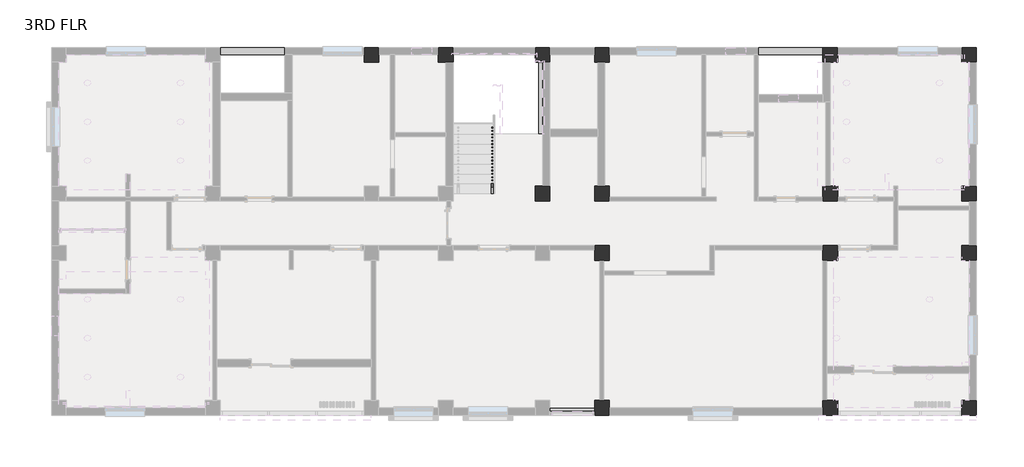
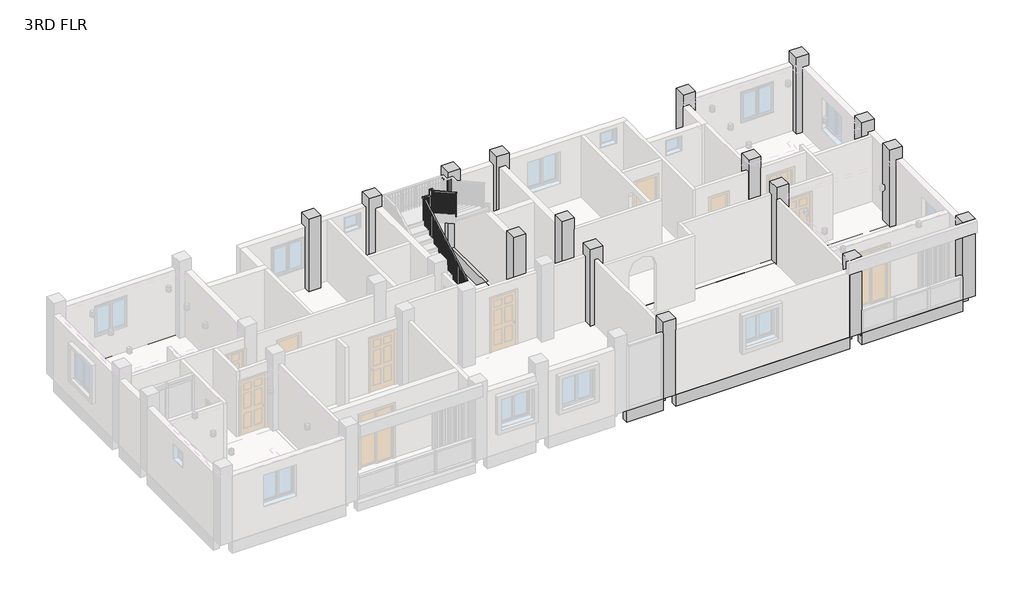
# One storey, part 4 of 5: 29 beams, 16 columns, 1 railing.
"""IFC4 building model written with IfcOpenShell, lengths in millimetres."""

from ifc_helpers import new_model, si_unit, frame, origin, place, context, project, spatial, polyline, outline, extrude, faceted_brep, element, save

model = new_model("IFC4")

# Units and contexts
model_context = context("Model", 3, world=origin())
ifc_project = project(units=[si_unit("LENGTHUNIT", "METRE", prefix="MILLI")], contexts=[model_context])

# Site, building, storey
site = spatial("IfcSite", under=ifc_project)
building = spatial("IfcBuilding", under=site)
storey = spatial("IfcBuildingStorey", under=building, Name="3RD FLR", Elevation=9448.8)

# Beams
placement = place(None, origin())
element("IfcBeam", 1, ObjectType="Concrete-Rectangular Beam : 9\" X 18\" BEAM", at=placement, inside=storey, context=model_context, shape_type="SweptSolid", body=[
    extrude(outline(polyline([(1310.3916602, -10887.8679047), (1310.3916602, -11116.4679047), (-61.2083398, -11116.4679047), (-61.2083398, -10887.8679047), (1310.3916602, -10887.8679047)])), frame((0.0, 0.0, 8991.6), z_axis=(0.0, 0.0, 1.0), x_axis=(1.0, 0.0, 0.0)), (0.0, 0.0, 1.0), 457.2),
])
element("IfcBeam", 2, ObjectType="Concrete-Rectangular Beam : 9\" X 18\" BEAM", at=placement, inside=storey, context=model_context, shape_type="SweptSolid", body=[
    extrude(outline(polyline([(1424.6916602, -6358.3794704), (1653.2916602, -6358.3794704), (1653.2916602, -10659.2679047), (1424.6916602, -10659.2679047), (1424.6916602, -6358.3794704)])), frame((0.0, 0.0, 8991.6), z_axis=(0.0, 0.0, 1.0), x_axis=(1.0, 0.0, 0.0)), (0.0, 0.0, 1.0), 457.2),
])
element("IfcBeam", 3, ObjectType="Concrete-Rectangular Beam : 9\" X 18\" BEAM", at=placement, inside=storey, context=model_context, shape_type="SweptSolid", body=[
    extrude(outline(polyline([(1424.6916602, -4529.5794704), (1653.2916602, -4529.5794704), (1653.2916602, -5901.1794704), (1424.6916602, -5901.1794704), (1424.6916602, -4529.5794704)])), frame((0.0, 0.0, 8991.6), z_axis=(0.0, 0.0, 1.0), x_axis=(1.0, 0.0, 0.0)), (0.0, 0.0, 1.0), 457.2),
])
element("IfcBeam", 4, ObjectType="Concrete-Rectangular Beam : 9\" X 18\" BEAM", at=placement, inside=storey, context=model_context, shape_type="SweptSolid", body=[
    extrude(outline(polyline([(8317.2128058, -10887.8679047), (8317.2128058, -11116.4679047), (1767.5916602, -11116.4679047), (1767.5916602, -10887.8679047), (8317.2128058, -10887.8679047)])), frame((0.0, 0.0, 8991.6), z_axis=(0.0, 0.0, 1.0), x_axis=(1.0, 0.0, 0.0)), (0.0, 0.0, 1.0), 457.2),
])
element("IfcBeam", 5, ObjectType="Concrete-Rectangular Beam : 9\" X 18\" BEAM", at=placement, inside=storey, context=model_context, shape_type="SweptSolid", body=[
    extrude(outline(polyline([(12584.4128058, -10887.8679047), (12584.4128058, -11116.4679047), (8774.4128058, -11116.4679047), (8774.4128058, -10887.8679047), (12584.4128058, -10887.8679047)])), frame((0.0, 0.0, 8991.6), z_axis=(0.0, 0.0, 1.0), x_axis=(1.0, 0.0, 0.0)), (0.0, 0.0, 1.0), 457.2),
])
element("IfcBeam", 6, ObjectType="Concrete-Rectangular Beam : 9\" X 18\" BEAM", at=placement, inside=storey, context=model_context, shape_type="SweptSolid", body=[
    extrude(outline(polyline([(12813.0128058, -6358.3794704), (13041.6128058, -6358.3794704), (13041.6128058, -10659.2679047), (12813.0128058, -10659.2679047), (12813.0128058, -6358.3794704)])), frame((0.0, 0.0, 8991.6), z_axis=(0.0, 0.0, 1.0), x_axis=(1.0, 0.0, 0.0)), (0.0, 0.0, 1.0), 457.2),
])
element("IfcBeam", 7, ObjectType="Concrete-Rectangular Beam : 9\" X 18\" BEAM", at=placement, inside=storey, context=model_context, shape_type="SweptSolid", body=[
    extrude(outline(polyline([(12813.0128058, -4529.5794704), (13041.6128058, -4529.5794704), (13041.6128058, -5901.1794704), (12813.0128058, -5901.1794704), (12813.0128058, -4529.5794704)])), frame((0.0, 0.0, 8991.6), z_axis=(0.0, 0.0, 1.0), x_axis=(1.0, 0.0, 0.0)), (0.0, 0.0, 1.0), 457.2),
])
element("IfcBeam", 8, ObjectType="Concrete-Rectangular Beam : 9\" X 18\" BEAM", at=placement, inside=storey, context=model_context, shape_type="SweptSolid", body=[
    extrude(outline(polyline([(12813.0128058, -262.3794704), (13041.6128058, -262.3794704), (13041.6128058, -4072.3794704), (12813.0128058, -4072.3794704), (12813.0128058, -262.3794704)])), frame((0.0, 0.0, 8991.6), z_axis=(0.0, 0.0, 1.0), x_axis=(1.0, 0.0, 0.0)), (0.0, 0.0, 1.0), 457.2),
])
element("IfcBeam", 9, ObjectType="Concrete-Rectangular Beam : 9\" X 18\" BEAM", at=placement, inside=storey, context=model_context, shape_type="SweptSolid", body=[
    extrude(outline(polyline([(8774.4128058, -33.7794704), (8774.4128058, 194.8205296), (12584.4128058, 194.8205296), (12584.4128058, -33.7794704), (8774.4128058, -33.7794704)])), frame((0.0, 0.0, 8991.6), z_axis=(0.0, 0.0, 1.0), x_axis=(1.0, 0.0, 0.0)), (0.0, 0.0, 1.0), 457.2),
])
element("IfcBeam", 10, ObjectType="Concrete-Rectangular Beam : 9\" X 18\" BEAM", at=placement, inside=storey, context=model_context, shape_type="SweptSolid", body=[
    extrude(outline(polyline([(1767.5916602, -33.7794704), (1767.5916602, 194.8205296), (8317.2128058, 194.8205296), (8317.2128058, -33.7794704), (1767.5916602, -33.7794704)])), frame((0.0, 0.0, 8991.6), z_axis=(0.0, 0.0, 1.0), x_axis=(1.0, 0.0, 0.0)), (0.0, 0.0, 1.0), 457.2),
])
element("IfcBeam", 11, ObjectType="Concrete-Rectangular Beam : 9\" X 18\" BEAM", at=placement, inside=storey, context=model_context, shape_type="SweptSolid", body=[
    extrude(outline(polyline([(-61.2083398, -33.7794704), (-61.2083398, 194.8205296), (1310.3916602, 194.8205296), (1310.3916602, -33.7794704), (-61.2083398, -33.7794704)])), frame((0.0, 0.0, 8991.6), z_axis=(0.0, 0.0, 1.0), x_axis=(1.0, 0.0, 0.0)), (0.0, 0.0, 1.0), 457.2),
])
element("IfcBeam", 12, ObjectType="Concrete-Rectangular Beam : 9\" X 18\" BEAM", at=placement, inside=storey, context=model_context, shape_type="SweptSolid", body=[
    extrude(outline(polyline([(-3029.5456086, -33.7794704), (-3029.5456086, 194.8205296), (-518.4083398, 194.8205296), (-518.4083398, -33.7794704), (-3029.5456086, -33.7794704)])), frame((0.0, 0.0, 8991.6), z_axis=(0.0, 0.0, 1.0), x_axis=(1.0, 0.0, 0.0)), (0.0, 0.0, 1.0), 457.2),
])
element("IfcBeam", 13, ObjectType="Concrete-Rectangular Beam : 9\" X 18\" BEAM", at=placement, inside=storey, context=model_context, shape_type="SweptSolid", body=[
    extrude(outline(polyline([(-5315.5456086, -33.7794704), (-5315.5456086, 194.8205296), (-3486.7456086, 194.8205296), (-3486.7456086, -33.7794704), (-5315.5456086, -33.7794704)])), frame((0.0, 0.0, 8991.6), z_axis=(0.0, 0.0, 1.0), x_axis=(1.0, 0.0, 0.0)), (0.0, 0.0, 1.0), 457.2),
])
element("IfcBeam", 14, ObjectType="Concrete-Rectangular Beam : 9\" X 18\" BEAM", at=placement, inside=storey, context=model_context, shape_type="SweptSolid", body=[
    extrude(outline(polyline([(-10192.3456086, -33.7794704), (-10192.3456086, 194.8205296), (-5772.7456086, 194.8205296), (-5772.7456086, -33.7794704), (-10192.3456086, -33.7794704)])), frame((0.0, 0.0, 8991.6), z_axis=(0.0, 0.0, 1.0), x_axis=(1.0, 0.0, 0.0)), (0.0, 0.0, 1.0), 457.2),
])
element("IfcBeam", 15, ObjectType="Concrete-Rectangular Beam : 9\" X 18\" BEAM", at=placement, inside=storey, context=model_context, shape_type="SweptSolid", body=[
    extrude(outline(polyline([(-14916.7456086, -33.7794704), (-14916.7456086, 194.8205296), (-10649.5456086, 194.8205296), (-10649.5456086, -33.7794704), (-14916.7456086, -33.7794704)])), frame((0.0, 0.0, 8991.6), z_axis=(0.0, 0.0, 1.0), x_axis=(1.0, 0.0, 0.0)), (0.0, 0.0, 1.0), 457.2),
])
element("IfcBeam", 16, ObjectType="Concrete-Rectangular Beam : 9\" X 18\" BEAM", at=placement, inside=storey, context=model_context, shape_type="SweptSolid", body=[
    extrude(outline(polyline([(-518.4083398, -4186.6794704), (-518.4083398, -4415.2794704), (-3029.5456086, -4415.2794704), (-3029.5456086, -4186.6794704), (-518.4083398, -4186.6794704)])), frame((0.0, 0.0, 8991.6), z_axis=(0.0, 0.0, 1.0), x_axis=(1.0, 0.0, 0.0)), (0.0, 0.0, 1.0), 457.2),
])
element("IfcBeam", 17, ObjectType="Concrete-Rectangular Beam : 9\" X 18\" BEAM", at=placement, inside=storey, context=model_context, shape_type="SweptSolid", body=[
    extrude(outline(polyline([(1310.3916602, -4186.6794704), (1310.3916602, -4415.2794704), (-61.2083398, -4415.2794704), (-61.2083398, -4186.6794704), (1310.3916602, -4186.6794704)])), frame((0.0, 0.0, 8991.6), z_axis=(0.0, 0.0, 1.0), x_axis=(1.0, 0.0, 0.0)), (0.0, 0.0, 1.0), 457.2),
])
element("IfcBeam", 18, ObjectType="Concrete-Rectangular Beam : 9\" X 18\" BEAM", at=placement, inside=storey, context=model_context, shape_type="SweptSolid", body=[
    extrude(outline(polyline([(1424.6916602, -262.3794704), (1653.2916602, -262.3794704), (1653.2916602, -4072.3794704), (1424.6916602, -4072.3794704), (1424.6916602, -262.3794704)])), frame((0.0, 0.0, 8991.6), z_axis=(0.0, 0.0, 1.0), x_axis=(1.0, 0.0, 0.0)), (0.0, 0.0, 1.0), 457.2),
])
element("IfcBeam", 19, ObjectType="Concrete-Rectangular Beam : 9\" X 18\" BEAM", at=placement, inside=storey, context=model_context, shape_type="SweptSolid", body=[
    extrude(outline(polyline([(-175.5083398, -4072.3794704), (-404.1083398, -4072.3794704), (-404.1083398, -262.3794704), (-175.5083398, -262.3794704), (-175.5083398, -4072.3794704)])), frame((0.0, 0.0, 8991.6), z_axis=(0.0, 0.0, 1.0), x_axis=(1.0, 0.0, 0.0)), (0.0, 0.0, 1.0), 457.2),
])
element("IfcBeam", 20, ObjectType="Concrete-Rectangular Beam : 9\" X 18\" BEAM", at=placement, inside=storey, context=model_context, shape_type="SweptSolid", body=[
    extrude(outline(polyline([(-3143.8456086, -4072.3794704), (-3372.4456086, -4072.3794704), (-3372.4456086, -262.3794704), (-3143.8456086, -262.3794704), (-3143.8456086, -4072.3794704)])), frame((0.0, 0.0, 8991.6), z_axis=(0.0, 0.0, 1.0), x_axis=(1.0, 0.0, 0.0)), (0.0, 0.0, 1.0), 457.2),
])
element("IfcBeam", 21, ObjectType="Concrete-Rectangular Beam : 9\" X 18\" BEAM", at=placement, inside=storey, context=model_context, shape_type="SweptSolid", body=[
    extrude(outline(polyline([(-5429.8456086, -4072.3794704), (-5658.4456086, -4072.3794704), (-5658.4456086, -262.3794704), (-5429.8456086, -262.3794704), (-5429.8456086, -4072.3794704)])), frame((0.0, 0.0, 8991.6), z_axis=(0.0, 0.0, 1.0), x_axis=(1.0, 0.0, 0.0)), (0.0, 0.0, 1.0), 457.2),
])
element("IfcBeam", 22, ObjectType="Concrete-Rectangular Beam : 9\" X 18\" BEAM", at=placement, inside=storey, context=model_context, shape_type="SweptSolid", body=[
    extrude(outline(polyline([(1310.3916602, -6015.4794704), (1310.3916602, -6244.0794704), (-61.2083398, -6244.0794704), (-61.2083398, -6015.4794704), (1310.3916602, -6015.4794704)])), frame((0.0, 0.0, 8991.6), z_axis=(0.0, 0.0, 1.0), x_axis=(1.0, 0.0, 0.0)), (0.0, 0.0, 1.0), 457.2),
])
element("IfcBeam", 23, ObjectType="Concrete-Rectangular Beam : 9\" X 18\" BEAM", at=placement, inside=storey, context=model_context, shape_type="SweptSolid", body=[
    extrude(outline(polyline([(8317.2128058, -4186.6794704), (8317.2128058, -4415.2794704), (1767.5916602, -4415.2794704), (1767.5916602, -4186.6794704), (8317.2128058, -4186.6794704)])), frame((0.0, 0.0, 8991.6), z_axis=(0.0, 0.0, 1.0), x_axis=(1.0, 0.0, 0.0)), (0.0, 0.0, 1.0), 457.2),
])
element("IfcBeam", 24, ObjectType="Concrete-Rectangular Beam : 9\" X 18\" BEAM", at=placement, inside=storey, context=model_context, shape_type="SweptSolid", body=[
    extrude(outline(polyline([(12584.4128058, -4186.6794704), (12584.4128058, -4415.2794704), (8774.4128058, -4415.2794704), (8774.4128058, -4186.6794704), (12584.4128058, -4186.6794704)])), frame((0.0, 0.0, 8991.6), z_axis=(0.0, 0.0, 1.0), x_axis=(1.0, 0.0, 0.0)), (0.0, 0.0, 1.0), 457.2),
])
element("IfcBeam", 25, ObjectType="Concrete-Rectangular Beam : 9\" X 18\" BEAM", at=placement, inside=storey, context=model_context, shape_type="SweptSolid", body=[
    extrude(outline(polyline([(8774.4128058, -6244.0794704), (8774.4128058, -6015.4794704), (12584.4128058, -6015.4794704), (12584.4128058, -6244.0794704), (8774.4128058, -6244.0794704)])), frame((0.0, 0.0, 8991.6), z_axis=(0.0, 0.0, 1.0), x_axis=(1.0, 0.0, 0.0)), (0.0, 0.0, 1.0), 457.2),
])
element("IfcBeam", 26, ObjectType="Concrete-Rectangular Beam : 9\" X 18\" BEAM", at=placement, inside=storey, context=model_context, shape_type="SweptSolid", body=[
    extrude(outline(polyline([(1767.5916602, -6244.0794704), (1767.5916602, -6015.4794704), (8317.2128058, -6015.4794704), (8317.2128058, -6244.0794704), (1767.5916602, -6244.0794704)])), frame((0.0, 0.0, 8991.6), z_axis=(0.0, 0.0, 1.0), x_axis=(1.0, 0.0, 0.0)), (0.0, 0.0, 1.0), 457.2),
])
element("IfcBeam", 27, ObjectType="Concrete-Rectangular Beam : 9\" X 18\" BEAM", at=placement, inside=storey, context=model_context, shape_type="SweptSolid", body=[
    extrude(outline(polyline([(8431.5128058, -6358.3794704), (8660.1128058, -6358.3794704), (8660.1128058, -10659.2679047), (8431.5128058, -10659.2679047), (8431.5128058, -6358.3794704)])), frame((0.0, 0.0, 8991.6), z_axis=(0.0, 0.0, 1.0), x_axis=(1.0, 0.0, 0.0)), (0.0, 0.0, 1.0), 457.2),
])
element("IfcBeam", 28, ObjectType="Concrete-Rectangular Beam : 9\" X 18\" BEAM", at=placement, inside=storey, context=model_context, shape_type="SweptSolid", body=[
    extrude(outline(polyline([(8431.5128058, -4529.5794704), (8660.1128058, -4529.5794704), (8660.1128058, -5901.1794704), (8431.5128058, -5901.1794704), (8431.5128058, -4529.5794704)])), frame((0.0, 0.0, 8991.6), z_axis=(0.0, 0.0, 1.0), x_axis=(1.0, 0.0, 0.0)), (0.0, 0.0, 1.0), 457.2),
])
element("IfcBeam", 29, ObjectType="Concrete-Rectangular Beam : 9\" X 18\" BEAM", at=placement, inside=storey, context=model_context, shape_type="SweptSolid", body=[
    extrude(outline(polyline([(8431.5128058, -262.3794704), (8660.1128058, -262.3794704), (8660.1128058, -4072.3794704), (8431.5128058, -4072.3794704), (8431.5128058, -262.3794704)])), frame((0.0, 0.0, 8991.6), z_axis=(0.0, 0.0, 1.0), x_axis=(1.0, 0.0, 0.0)), (0.0, 0.0, 1.0), 457.2),
])

# Columns
element("IfcColumn", 30, ObjectType="Concrete-Rectangular-Column : COLUMN 18\" X 18\"", at=placement, inside=storey, context=model_context, shape_type="SweptSolid", body=[
    extrude(outline(polyline([(-5315.5456086, 194.8205296), (-5315.5456086, -262.3794704), (-5772.7456086, -262.3794704), (-5772.7456086, 194.8205296), (-5315.5456086, 194.8205296)])), frame((0.0, 0.0, 9448.8), z_axis=(0.0, 0.0, 1.0), x_axis=(1.0, 0.0, 0.0)), (0.0, 0.0, 1.0), 3048.0),
])
element("IfcColumn", 31, ObjectType="Concrete-Rectangular-Column : COLUMN 18\" X 18\"", at=placement, inside=storey, context=model_context, shape_type="SweptSolid", body=[
    extrude(outline(polyline([(-3029.5456086, 194.8205296), (-3029.5456086, -262.3794704), (-3486.7456086, -262.3794704), (-3486.7456086, 194.8205296), (-3029.5456086, 194.8205296)])), frame((0.0, 0.0, 9448.8), z_axis=(0.0, 0.0, 1.0), x_axis=(1.0, 0.0, 0.0)), (0.0, 0.0, 1.0), 3048.0),
])
element("IfcColumn", 32, ObjectType="Concrete-Rectangular-Column : COLUMN 18\" X 18\"", at=placement, inside=storey, context=model_context, shape_type="SweptSolid", body=[
    extrude(outline(polyline([(-61.2083398, 194.8205296), (-61.2083398, -262.3794704), (-518.4083398, -262.3794704), (-518.4083398, 194.8205296), (-61.2083398, 194.8205296)])), frame((0.0, 0.0, 9448.8), z_axis=(0.0, 0.0, 1.0), x_axis=(1.0, 0.0, 0.0)), (0.0, 0.0, 1.0), 3048.0),
])
element("IfcColumn", 33, ObjectType="Concrete-Rectangular-Column : COLUMN 18\" X 18\"", at=placement, inside=storey, context=model_context, shape_type="SweptSolid", body=[
    extrude(outline(polyline([(1767.5916602, 194.8205296), (1767.5916602, -262.3794704), (1310.3916602, -262.3794704), (1310.3916602, 194.8205296), (1767.5916602, 194.8205296)])), frame((0.0, 0.0, 9448.8), z_axis=(0.0, 0.0, 1.0), x_axis=(1.0, 0.0, 0.0)), (0.0, 0.0, 1.0), 3048.0),
])
element("IfcColumn", 34, ObjectType="Concrete-Rectangular-Column : COLUMN 18\" X 18\"", at=placement, inside=storey, context=model_context, shape_type="SweptSolid", body=[
    extrude(outline(polyline([(8774.4128058, 194.8205296), (8774.4128058, -262.3794704), (8317.2128058, -262.3794704), (8317.2128058, 194.8205296), (8774.4128058, 194.8205296)])), frame((0.0, 0.0, 9448.8), z_axis=(0.0, 0.0, 1.0), x_axis=(1.0, 0.0, 0.0)), (0.0, 0.0, 1.0), 3048.0),
])
element("IfcColumn", 35, ObjectType="Concrete-Rectangular-Column : COLUMN 18\" X 18\"", at=placement, inside=storey, context=model_context, shape_type="SweptSolid", body=[
    extrude(outline(polyline([(13041.6128058, 194.8205296), (13041.6128058, -262.3794704), (12584.4128058, -262.3794704), (12584.4128058, 194.8205296), (13041.6128058, 194.8205296)])), frame((0.0, 0.0, 9448.8), z_axis=(0.0, 0.0, 1.0), x_axis=(1.0, 0.0, 0.0)), (0.0, 0.0, 1.0), 3048.0),
])
element("IfcColumn", 36, ObjectType="Concrete-Rectangular-Column : COLUMN 18\" X 18\"", at=placement, inside=storey, context=model_context, shape_type="SweptSolid", body=[
    extrude(outline(polyline([(13041.6128058, -4072.3794704), (13041.6128058, -4529.5794704), (12584.4128058, -4529.5794704), (12584.4128058, -4072.3794704), (13041.6128058, -4072.3794704)])), frame((0.0, 0.0, 9448.8), z_axis=(0.0, 0.0, 1.0), x_axis=(1.0, 0.0, 0.0)), (0.0, 0.0, 1.0), 3048.0),
])
element("IfcColumn", 37, ObjectType="Concrete-Rectangular-Column : COLUMN 18\" X 18\"", at=placement, inside=storey, context=model_context, shape_type="SweptSolid", body=[
    extrude(outline(polyline([(13041.6128058, -5901.1794704), (13041.6128058, -6358.3794704), (12584.4128058, -6358.3794704), (12584.4128058, -5901.1794704), (13041.6128058, -5901.1794704)])), frame((0.0, 0.0, 9448.8), z_axis=(0.0, 0.0, 1.0), x_axis=(1.0, 0.0, 0.0)), (0.0, 0.0, 1.0), 3048.0),
])
element("IfcColumn", 38, ObjectType="Concrete-Rectangular-Column : COLUMN 18\" X 18\"", at=placement, inside=storey, context=model_context, shape_type="SweptSolid", body=[
    extrude(outline(polyline([(13041.6128058, -10659.2679047), (13041.6128058, -11116.4679047), (12584.4128058, -11116.4679047), (12584.4128058, -10659.2679047), (13041.6128058, -10659.2679047)])), frame((0.0, 0.0, 9448.8), z_axis=(0.0, 0.0, 1.0), x_axis=(1.0, 0.0, 0.0)), (0.0, 0.0, 1.0), 3048.0),
])
element("IfcColumn", 39, ObjectType="Concrete-Rectangular-Column : COLUMN 18\" X 18\"", at=placement, inside=storey, context=model_context, shape_type="SweptSolid", body=[
    extrude(outline(polyline([(8774.4128058, -10659.2679047), (8774.4128058, -11116.4679047), (8317.2128058, -11116.4679047), (8317.2128058, -10659.2679047), (8774.4128058, -10659.2679047)])), frame((0.0, 0.0, 9448.8), z_axis=(0.0, 0.0, 1.0), x_axis=(1.0, 0.0, 0.0)), (0.0, 0.0, 1.0), 3048.0),
])
element("IfcColumn", 40, ObjectType="Concrete-Rectangular-Column : COLUMN 18\" X 18\"", at=placement, inside=storey, context=model_context, shape_type="SweptSolid", body=[
    extrude(outline(polyline([(1767.5916602, -10659.2679047), (1767.5916602, -11116.4679047), (1310.3916602, -11116.4679047), (1310.3916602, -10659.2679047), (1767.5916602, -10659.2679047)])), frame((0.0, 0.0, 9448.8), z_axis=(0.0, 0.0, 1.0), x_axis=(1.0, 0.0, 0.0)), (0.0, 0.0, 1.0), 3048.0),
])
element("IfcColumn", 41, ObjectType="Concrete-Rectangular-Column : COLUMN 18\" X 18\"", at=placement, inside=storey, context=model_context, shape_type="SweptSolid", body=[
    extrude(outline(polyline([(-61.2083398, -4072.3794704), (-61.2083398, -4529.5794704), (-518.4083398, -4529.5794704), (-518.4083398, -4072.3794704), (-61.2083398, -4072.3794704)])), frame((0.0, 0.0, 9448.8), z_axis=(0.0, 0.0, 1.0), x_axis=(1.0, 0.0, 0.0)), (0.0, 0.0, 1.0), 3048.0),
])
element("IfcColumn", 42, ObjectType="Concrete-Rectangular-Column : COLUMN 18\" X 18\"", at=placement, inside=storey, context=model_context, shape_type="SweptSolid", body=[
    extrude(outline(polyline([(1767.5916602, -4072.3794704), (1767.5916602, -4529.5794704), (1310.3916602, -4529.5794704), (1310.3916602, -4072.3794704), (1767.5916602, -4072.3794704)])), frame((0.0, 0.0, 9448.8), z_axis=(0.0, 0.0, 1.0), x_axis=(1.0, 0.0, 0.0)), (0.0, 0.0, 1.0), 3048.0),
])
element("IfcColumn", 43, ObjectType="Concrete-Rectangular-Column : COLUMN 18\" X 18\"", at=placement, inside=storey, context=model_context, shape_type="SweptSolid", body=[
    extrude(outline(polyline([(8774.4128058, -4072.3794704), (8774.4128058, -4529.5794704), (8317.2128058, -4529.5794704), (8317.2128058, -4072.3794704), (8774.4128058, -4072.3794704)])), frame((0.0, 0.0, 9448.8), z_axis=(0.0, 0.0, 1.0), x_axis=(1.0, 0.0, 0.0)), (0.0, 0.0, 1.0), 3048.0),
])
element("IfcColumn", 44, ObjectType="Concrete-Rectangular-Column : COLUMN 18\" X 18\"", at=placement, inside=storey, context=model_context, shape_type="SweptSolid", body=[
    extrude(outline(polyline([(8774.4128058, -5901.1794704), (8774.4128058, -6358.3794704), (8317.2128058, -6358.3794704), (8317.2128058, -5901.1794704), (8774.4128058, -5901.1794704)])), frame((0.0, 0.0, 9448.8), z_axis=(0.0, 0.0, 1.0), x_axis=(1.0, 0.0, 0.0)), (0.0, 0.0, 1.0), 3048.0),
])
element("IfcColumn", 45, ObjectType="Concrete-Rectangular-Column : COLUMN 18\" X 18\"", at=placement, inside=storey, context=model_context, shape_type="SweptSolid", body=[
    extrude(outline(polyline([(1767.5916602, -5901.1794704), (1767.5916602, -6358.3794704), (1310.3916602, -6358.3794704), (1310.3916602, -5901.1794704), (1767.5916602, -5901.1794704)])), frame((0.0, 0.0, 9448.8), z_axis=(0.0, 0.0, 1.0), x_axis=(1.0, 0.0, 0.0)), (0.0, 0.0, 1.0), 3048.0),
])

# Railing
element("IfcRailing", 46, ObjectType="Handrail - Rectangular", at=placement, inside=storey, context=model_context, shape_type="SolidModel", body=[
    faceted_brep([(-1861.1456086, -4300.9794704, 10532.5333333), (-1861.1456086, -4300.9794704, 10474.420221), (-1810.3456086, -4300.9794704, 10474.420221), (-1810.3456086, -4300.9794704, 10532.5333333), (-1861.1456086, -1024.3794704, 12352.8666667), (-1861.1456086, -973.5794704, 12322.9757765), (-1810.3456086, -973.5794704, 12322.9757765), (-1810.3456086, -1024.3794704, 12352.8666667), (-1861.1456086, -1024.3794704, 12395.2), (-1861.1456086, -973.5794704, 12344.4), (-1810.3456086, -973.5794704, 12344.4), (-1810.3456086, -1024.3794704, 12395.2), (-1861.1456086, -897.3794704, 12395.2), (-1861.1456086, -897.3794704, 12344.4), (-1810.3456086, -948.1794704, 12344.4), (-1810.3456086, -948.1794704, 12395.2), (-1734.1456086, -897.3794704, 12395.2), (-1734.1456086, -897.3794704, 12344.4), (-1734.1456086, -948.1794704, 12344.4), (-1734.1456086, -948.1794704, 12395.2), (-1610.6083398, -897.3794704, 12395.2), (-1559.8083398, -897.3794704, 12344.4), (-1559.8083398, -948.1794704, 12344.4), (-1610.6083398, -948.1794704, 12395.2), (-1610.6083398, -897.3794704, 12606.8666667), (-1559.8083398, -897.3794704, 12556.0666667), (-1559.8083398, -948.1794704, 12556.0666667), (-1610.6083398, -948.1794704, 12606.8666667), (-1483.6083398, -897.3794704, 12606.8666667), (-1483.6083398, -897.3794704, 12556.0666667), (-1534.4083398, -948.1794704, 12556.0666667), (-1534.4083398, -948.1794704, 12606.8666667), (-1483.6083398, -1024.3794704, 12606.8666667), (-1483.6083398, -1037.5430727, 12556.0666667), (-1534.4083398, -1037.5430727, 12556.0666667), (-1534.4083398, -1024.3794704, 12606.8666667), (-1483.6083398, -2472.1794704, 13411.2), (-1534.4083398, -2472.1794704, 13411.2), (-1534.4083398, -2472.1794704, 13353.0868876), (-1483.6083398, -2472.1794704, 13353.0868876)], [[[0, 1, 2, 3]], [[1, 0, 4, 5]], [[2, 1, 5, 6]], [[3, 2, 6, 7]], [[0, 3, 7, 4]], [[5, 4, 8, 9]], [[6, 5, 9, 10]], [[7, 6, 10, 11]], [[4, 7, 11, 8]], [[9, 8, 12, 13]], [[10, 9, 13, 14]], [[11, 10, 14, 15]], [[8, 11, 15, 12]], [[13, 12, 16, 17]], [[14, 13, 17, 18]], [[15, 14, 18, 19]], [[12, 15, 19, 16]], [[17, 16, 20, 21]], [[18, 17, 21, 22]], [[19, 18, 22, 23]], [[16, 19, 23, 20]], [[21, 20, 24, 25]], [[22, 21, 25, 26]], [[23, 22, 26, 27]], [[20, 23, 27, 24]], [[25, 24, 28, 29]], [[26, 25, 29, 30]], [[27, 26, 30, 31]], [[24, 27, 31, 28]], [[29, 28, 32, 33]], [[30, 29, 33, 34]], [[31, 30, 34, 35]], [[28, 31, 35, 32]], [[36, 37, 38, 39]], [[33, 32, 36, 39]], [[34, 33, 39, 38]], [[35, 34, 38, 37]], [[32, 35, 37, 36]]]),
    extrude(outline(polyline([(-2456.3044704, 13344.2674432), (-2437.2544704, 13333.6841099), (-2437.2544704, 12327.4666667), (-2456.3044704, 12327.4666667), (-2456.3044704, 13344.2674432)])), frame((-1518.5333398, 0.0, 0.0), z_axis=(1.0, 0.0, 0.0), x_axis=(0.0, 1.0, 0.0)), (0.0, 0.0, 1.0), 19.05),
    extrude(outline(polyline([(-2354.7044704, 13287.8229988), (-2335.6544704, 13277.2396654), (-2335.6544704, 12327.4666667), (-2354.7044704, 12327.4666667), (-2354.7044704, 13287.8229988)])), frame((-1518.5333398, 0.0, 0.0), z_axis=(1.0, 0.0, 0.0), x_axis=(0.0, 1.0, 0.0)), (0.0, 0.0, 1.0), 19.05),
    extrude(outline(polyline([(-2253.1044704, 13231.3785543), (-2234.0544704, 13220.795221), (-2234.0544704, 12327.4666667), (-2253.1044704, 12327.4666667), (-2253.1044704, 13231.3785543)])), frame((-1518.5333398, 0.0, 0.0), z_axis=(1.0, 0.0, 0.0), x_axis=(0.0, 1.0, 0.0)), (0.0, 0.0, 1.0), 19.05),
    extrude(outline(polyline([(-2151.5044704, 13174.9341099), (-2132.4544704, 13164.3507765), (-2132.4544704, 12158.1333333), (-2151.5044704, 12158.1333333), (-2151.5044704, 13174.9341099)])), frame((-1518.5333398, 0.0, 0.0), z_axis=(1.0, 0.0, 0.0), x_axis=(0.0, 1.0, 0.0)), (0.0, 0.0, 1.0), 19.05),
    extrude(outline(polyline([(-2049.9044704, 13118.4896654), (-2030.8544704, 13107.9063321), (-2030.8544704, 12158.1333333), (-2049.9044704, 12158.1333333), (-2049.9044704, 13118.4896654)])), frame((-1518.5333398, 0.0, 0.0), z_axis=(1.0, 0.0, 0.0), x_axis=(0.0, 1.0, 0.0)), (0.0, 0.0, 1.0), 19.05),
    extrude(outline(polyline([(-1948.3044704, 13062.045221), (-1929.2544704, 13051.4618876), (-1929.2544704, 12158.1333333), (-1948.3044704, 12158.1333333), (-1948.3044704, 13062.045221)])), frame((-1518.5333398, 0.0, 0.0), z_axis=(1.0, 0.0, 0.0), x_axis=(0.0, 1.0, 0.0)), (0.0, 0.0, 1.0), 19.05),
    extrude(outline(polyline([(-1846.7044704, 13005.6007765), (-1827.6544704, 12995.0174432), (-1827.6544704, 11988.8), (-1846.7044704, 11988.8), (-1846.7044704, 13005.6007765)])), frame((-1518.5333398, 0.0, 0.0), z_axis=(1.0, 0.0, 0.0), x_axis=(0.0, 1.0, 0.0)), (0.0, 0.0, 1.0), 19.05),
    extrude(outline(polyline([(-1745.1044704, 12949.1563321), (-1726.0544704, 12938.5729988), (-1726.0544704, 11988.8), (-1745.1044704, 11988.8), (-1745.1044704, 12949.1563321)])), frame((-1518.5333398, 0.0, 0.0), z_axis=(1.0, 0.0, 0.0), x_axis=(0.0, 1.0, 0.0)), (0.0, 0.0, 1.0), 19.05),
    extrude(outline(polyline([(-1643.5044704, 12892.7118876), (-1624.4544704, 12882.1285543), (-1624.4544704, 11988.8), (-1643.5044704, 11988.8), (-1643.5044704, 12892.7118876)])), frame((-1518.5333398, 0.0, 0.0), z_axis=(1.0, 0.0, 0.0), x_axis=(0.0, 1.0, 0.0)), (0.0, 0.0, 1.0), 19.05),
    extrude(outline(polyline([(-1541.9044704, 12836.2674432), (-1522.8544704, 12825.6841099), (-1522.8544704, 11819.4666667), (-1541.9044704, 11819.4666667), (-1541.9044704, 12836.2674432)])), frame((-1518.5333398, 0.0, 0.0), z_axis=(1.0, 0.0, 0.0), x_axis=(0.0, 1.0, 0.0)), (0.0, 0.0, 1.0), 19.05),
    extrude(outline(polyline([(-1440.3044704, 12779.8229988), (-1421.2544704, 12769.2396654), (-1421.2544704, 11819.4666667), (-1440.3044704, 11819.4666667), (-1440.3044704, 12779.8229988)])), frame((-1518.5333398, 0.0, 0.0), z_axis=(1.0, 0.0, 0.0), x_axis=(0.0, 1.0, 0.0)), (0.0, 0.0, 1.0), 19.05),
    extrude(outline(polyline([(-1338.7044704, 12723.3785543), (-1319.6544704, 12712.795221), (-1319.6544704, 11819.4666667), (-1338.7044704, 11819.4666667), (-1338.7044704, 12723.3785543)])), frame((-1518.5333398, 0.0, 0.0), z_axis=(1.0, 0.0, 0.0), x_axis=(0.0, 1.0, 0.0)), (0.0, 0.0, 1.0), 19.05),
    extrude(outline(polyline([(-1237.1044704, 12666.9341099), (-1218.0544704, 12656.3507765), (-1218.0544704, 11650.1333333), (-1237.1044704, 11650.1333333), (-1237.1044704, 12666.9341099)])), frame((-1518.5333398, 0.0, 0.0), z_axis=(1.0, 0.0, 0.0), x_axis=(0.0, 1.0, 0.0)), (0.0, 0.0, 1.0), 19.05),
    extrude(outline(polyline([(-1135.5044704, 12610.4896654), (-1116.4544704, 12599.9063321), (-1116.4544704, 11650.1333333), (-1135.5044704, 11650.1333333), (-1135.5044704, 12610.4896654)])), frame((-1518.5333398, 0.0, 0.0), z_axis=(1.0, 0.0, 0.0), x_axis=(0.0, 1.0, 0.0)), (0.0, 0.0, 1.0), 19.05),
    extrude(outline(polyline([(-1033.9044704, 12554.045221), (-1014.8544704, 12543.4618876), (-1014.8544704, 11650.1333333), (-1033.9044704, 11650.1333333), (-1033.9044704, 12554.045221)])), frame((-1518.5333398, 0.0, 0.0), z_axis=(1.0, 0.0, 0.0), x_axis=(0.0, 1.0, 0.0)), (0.0, 0.0, 1.0), 19.05),
    extrude(outline(polyline([(-1540.4706086, -932.3044704), (-1540.4706086, -913.2544704), (-1521.4206086, -913.2544704), (-1521.4206086, -932.3044704), (-1540.4706086, -932.3044704)])), frame((0.0, 0.0, 11480.8), z_axis=(0.0, 0.0, 1.0), x_axis=(1.0, 0.0, 0.0)), (0.0, 0.0, 1.0), 1075.2666667),
    extrude(outline(polyline([(-1642.0706086, -932.3044704), (-1642.0706086, -913.2544704), (-1623.0206086, -913.2544704), (-1623.0206086, -932.3044704), (-1642.0706086, -932.3044704)])), frame((0.0, 0.0, 11480.8), z_axis=(0.0, 0.0, 1.0), x_axis=(1.0, 0.0, 0.0)), (0.0, 0.0, 1.0), 863.6),
    extrude(outline(polyline([(-1743.6706086, -932.3044704), (-1743.6706086, -913.2544704), (-1724.6206086, -913.2544704), (-1724.6206086, -932.3044704), (-1743.6706086, -932.3044704)])), frame((0.0, 0.0, 11480.8), z_axis=(0.0, 0.0, 1.0), x_axis=(1.0, 0.0, 0.0)), (0.0, 0.0, 1.0), 863.6),
    extrude(outline(polyline([(-1826.2206086, -957.7044704), (-1845.2706086, -957.7044704), (-1845.2706086, -938.6544704), (-1826.2206086, -938.6544704), (-1826.2206086, -957.7044704)])), frame((0.0, 0.0, 11480.8), z_axis=(0.0, 0.0, 1.0), x_axis=(1.0, 0.0, 0.0)), (0.0, 0.0, 1.0), 863.6),
    extrude(outline(polyline([(-1059.3044704, 12275.3507765), (-1040.2544704, 12285.9341099), (-1040.2544704, 11311.4666667), (-1059.3044704, 11311.4666667), (-1059.3044704, 12275.3507765)])), frame((-1845.2706086, 0.0, 0.0), z_axis=(1.0, 0.0, 0.0), x_axis=(0.0, 1.0, 0.0)), (0.0, 0.0, 1.0), 19.05),
    extrude(outline(polyline([(-1160.9044704, 12218.9063321), (-1141.8544704, 12229.4896654), (-1141.8544704, 11311.4666667), (-1160.9044704, 11311.4666667), (-1160.9044704, 12218.9063321)])), frame((-1845.2706086, 0.0, 0.0), z_axis=(1.0, 0.0, 0.0), x_axis=(0.0, 1.0, 0.0)), (0.0, 0.0, 1.0), 19.05),
    extrude(outline(polyline([(-1262.5044704, 12162.4618876), (-1243.4544704, 12173.045221), (-1243.4544704, 11311.4666667), (-1262.5044704, 11311.4666667), (-1262.5044704, 12162.4618876)])), frame((-1845.2706086, 0.0, 0.0), z_axis=(1.0, 0.0, 0.0), x_axis=(0.0, 1.0, 0.0)), (0.0, 0.0, 1.0), 19.05),
    extrude(outline(polyline([(-1364.1044704, 12106.0174432), (-1345.0544704, 12116.6007765), (-1345.0544704, 11142.1333333), (-1364.1044704, 11142.1333333), (-1364.1044704, 12106.0174432)])), frame((-1845.2706086, 0.0, 0.0), z_axis=(1.0, 0.0, 0.0), x_axis=(0.0, 1.0, 0.0)), (0.0, 0.0, 1.0), 19.05),
    extrude(outline(polyline([(-1465.7044704, 12049.5729988), (-1446.6544704, 12060.1563321), (-1446.6544704, 11142.1333333), (-1465.7044704, 11142.1333333), (-1465.7044704, 12049.5729988)])), frame((-1845.2706086, 0.0, 0.0), z_axis=(1.0, 0.0, 0.0), x_axis=(0.0, 1.0, 0.0)), (0.0, 0.0, 1.0), 19.05),
    extrude(outline(polyline([(-1567.3044704, 11993.1285543), (-1548.2544704, 12003.7118876), (-1548.2544704, 11142.1333333), (-1567.3044704, 11142.1333333), (-1567.3044704, 11993.1285543)])), frame((-1845.2706086, 0.0, 0.0), z_axis=(1.0, 0.0, 0.0), x_axis=(0.0, 1.0, 0.0)), (0.0, 0.0, 1.0), 19.05),
    extrude(outline(polyline([(-1668.9044704, 11936.6841099), (-1649.8544704, 11947.2674432), (-1649.8544704, 10972.8), (-1668.9044704, 10972.8), (-1668.9044704, 11936.6841099)])), frame((-1845.2706086, 0.0, 0.0), z_axis=(1.0, 0.0, 0.0), x_axis=(0.0, 1.0, 0.0)), (0.0, 0.0, 1.0), 19.05),
    extrude(outline(polyline([(-1770.5044704, 11880.2396654), (-1751.4544704, 11890.8229988), (-1751.4544704, 10972.8), (-1770.5044704, 10972.8), (-1770.5044704, 11880.2396654)])), frame((-1845.2706086, 0.0, 0.0), z_axis=(1.0, 0.0, 0.0), x_axis=(0.0, 1.0, 0.0)), (0.0, 0.0, 1.0), 19.05),
    extrude(outline(polyline([(-1872.1044704, 11823.795221), (-1853.0544704, 11834.3785543), (-1853.0544704, 10972.8), (-1872.1044704, 10972.8), (-1872.1044704, 11823.795221)])), frame((-1845.2706086, 0.0, 0.0), z_axis=(1.0, 0.0, 0.0), x_axis=(0.0, 1.0, 0.0)), (0.0, 0.0, 1.0), 19.05),
    extrude(outline(polyline([(-1973.7044704, 11767.3507765), (-1954.6544704, 11777.9341099), (-1954.6544704, 10803.4666667), (-1973.7044704, 10803.4666667), (-1973.7044704, 11767.3507765)])), frame((-1845.2706086, 0.0, 0.0), z_axis=(1.0, 0.0, 0.0), x_axis=(0.0, 1.0, 0.0)), (0.0, 0.0, 1.0), 19.05),
    extrude(outline(polyline([(-2075.3044704, 11710.9063321), (-2056.2544704, 11721.4896654), (-2056.2544704, 10803.4666667), (-2075.3044704, 10803.4666667), (-2075.3044704, 11710.9063321)])), frame((-1845.2706086, 0.0, 0.0), z_axis=(1.0, 0.0, 0.0), x_axis=(0.0, 1.0, 0.0)), (0.0, 0.0, 1.0), 19.05),
    extrude(outline(polyline([(-2176.9044704, 11654.4618876), (-2157.8544704, 11665.045221), (-2157.8544704, 10803.4666667), (-2176.9044704, 10803.4666667), (-2176.9044704, 11654.4618876)])), frame((-1845.2706086, 0.0, 0.0), z_axis=(1.0, 0.0, 0.0), x_axis=(0.0, 1.0, 0.0)), (0.0, 0.0, 1.0), 19.05),
    extrude(outline(polyline([(-2278.5044704, 11598.0174432), (-2259.4544704, 11608.6007765), (-2259.4544704, 10634.1333333), (-2278.5044704, 10634.1333333), (-2278.5044704, 11598.0174432)])), frame((-1845.2706086, 0.0, 0.0), z_axis=(1.0, 0.0, 0.0), x_axis=(0.0, 1.0, 0.0)), (0.0, 0.0, 1.0), 19.05),
    extrude(outline(polyline([(-2380.1044704, 11541.5729988), (-2361.0544704, 11552.1563321), (-2361.0544704, 10634.1333333), (-2380.1044704, 10634.1333333), (-2380.1044704, 11541.5729988)])), frame((-1845.2706086, 0.0, 0.0), z_axis=(1.0, 0.0, 0.0), x_axis=(0.0, 1.0, 0.0)), (0.0, 0.0, 1.0), 19.05),
    extrude(outline(polyline([(-2481.7044704, 11485.1285543), (-2462.6544704, 11495.7118876), (-2462.6544704, 10634.1333333), (-2481.7044704, 10634.1333333), (-2481.7044704, 11485.1285543)])), frame((-1845.2706086, 0.0, 0.0), z_axis=(1.0, 0.0, 0.0), x_axis=(0.0, 1.0, 0.0)), (0.0, 0.0, 1.0), 19.05),
    extrude(outline(polyline([(-2583.3044704, 11428.6841099), (-2564.2544704, 11439.2674432), (-2564.2544704, 10464.8), (-2583.3044704, 10464.8), (-2583.3044704, 11428.6841099)])), frame((-1845.2706086, 0.0, 0.0), z_axis=(1.0, 0.0, 0.0), x_axis=(0.0, 1.0, 0.0)), (0.0, 0.0, 1.0), 19.05),
    extrude(outline(polyline([(-2684.9044704, 11372.2396654), (-2665.8544704, 11382.8229988), (-2665.8544704, 10464.8), (-2684.9044704, 10464.8), (-2684.9044704, 11372.2396654)])), frame((-1845.2706086, 0.0, 0.0), z_axis=(1.0, 0.0, 0.0), x_axis=(0.0, 1.0, 0.0)), (0.0, 0.0, 1.0), 19.05),
    extrude(outline(polyline([(-2786.5044704, 11315.795221), (-2767.4544704, 11326.3785543), (-2767.4544704, 10464.8), (-2786.5044704, 10464.8), (-2786.5044704, 11315.795221)])), frame((-1845.2706086, 0.0, 0.0), z_axis=(1.0, 0.0, 0.0), x_axis=(0.0, 1.0, 0.0)), (0.0, 0.0, 1.0), 19.05),
    extrude(outline(polyline([(-2888.1044704, 11259.3507765), (-2869.0544704, 11269.9341099), (-2869.0544704, 10295.4666667), (-2888.1044704, 10295.4666667), (-2888.1044704, 11259.3507765)])), frame((-1845.2706086, 0.0, 0.0), z_axis=(1.0, 0.0, 0.0), x_axis=(0.0, 1.0, 0.0)), (0.0, 0.0, 1.0), 19.05),
    extrude(outline(polyline([(-2989.7044704, 11202.9063321), (-2970.6544704, 11213.4896654), (-2970.6544704, 10295.4666667), (-2989.7044704, 10295.4666667), (-2989.7044704, 11202.9063321)])), frame((-1845.2706086, 0.0, 0.0), z_axis=(1.0, 0.0, 0.0), x_axis=(0.0, 1.0, 0.0)), (0.0, 0.0, 1.0), 19.05),
    extrude(outline(polyline([(-3091.3044704, 11146.4618876), (-3072.2544704, 11157.045221), (-3072.2544704, 10295.4666667), (-3091.3044704, 10295.4666667), (-3091.3044704, 11146.4618876)])), frame((-1845.2706086, 0.0, 0.0), z_axis=(1.0, 0.0, 0.0), x_axis=(0.0, 1.0, 0.0)), (0.0, 0.0, 1.0), 19.05),
    extrude(outline(polyline([(-3192.9044704, 11090.0174432), (-3173.8544704, 11100.6007765), (-3173.8544704, 10126.1333333), (-3192.9044704, 10126.1333333), (-3192.9044704, 11090.0174432)])), frame((-1845.2706086, 0.0, 0.0), z_axis=(1.0, 0.0, 0.0), x_axis=(0.0, 1.0, 0.0)), (0.0, 0.0, 1.0), 19.05),
    extrude(outline(polyline([(-3294.5044704, 11033.5729988), (-3275.4544704, 11044.1563321), (-3275.4544704, 10126.1333333), (-3294.5044704, 10126.1333333), (-3294.5044704, 11033.5729988)])), frame((-1845.2706086, 0.0, 0.0), z_axis=(1.0, 0.0, 0.0), x_axis=(0.0, 1.0, 0.0)), (0.0, 0.0, 1.0), 19.05),
    extrude(outline(polyline([(-3396.1044704, 10977.1285543), (-3377.0544704, 10987.7118876), (-3377.0544704, 10126.1333333), (-3396.1044704, 10126.1333333), (-3396.1044704, 10977.1285543)])), frame((-1845.2706086, 0.0, 0.0), z_axis=(1.0, 0.0, 0.0), x_axis=(0.0, 1.0, 0.0)), (0.0, 0.0, 1.0), 19.05),
    extrude(outline(polyline([(-3497.7044704, 10920.6841099), (-3478.6544704, 10931.2674432), (-3478.6544704, 9956.8), (-3497.7044704, 9956.8), (-3497.7044704, 10920.6841099)])), frame((-1845.2706086, 0.0, 0.0), z_axis=(1.0, 0.0, 0.0), x_axis=(0.0, 1.0, 0.0)), (0.0, 0.0, 1.0), 19.05),
    extrude(outline(polyline([(-3599.3044704, 10864.2396654), (-3580.2544704, 10874.8229988), (-3580.2544704, 9956.8), (-3599.3044704, 9956.8), (-3599.3044704, 10864.2396654)])), frame((-1845.2706086, 0.0, 0.0), z_axis=(1.0, 0.0, 0.0), x_axis=(0.0, 1.0, 0.0)), (0.0, 0.0, 1.0), 19.05),
    extrude(outline(polyline([(-3700.9044704, 10807.795221), (-3681.8544704, 10818.3785543), (-3681.8544704, 9956.8), (-3700.9044704, 9956.8), (-3700.9044704, 10807.795221)])), frame((-1845.2706086, 0.0, 0.0), z_axis=(1.0, 0.0, 0.0), x_axis=(0.0, 1.0, 0.0)), (0.0, 0.0, 1.0), 19.05),
    extrude(outline(polyline([(-3802.5044704, 10751.3507765), (-3783.4544704, 10761.9341099), (-3783.4544704, 9787.4666667), (-3802.5044704, 9787.4666667), (-3802.5044704, 10751.3507765)])), frame((-1845.2706086, 0.0, 0.0), z_axis=(1.0, 0.0, 0.0), x_axis=(0.0, 1.0, 0.0)), (0.0, 0.0, 1.0), 19.05),
    extrude(outline(polyline([(-3904.1044704, 10694.9063321), (-3885.0544704, 10705.4896654), (-3885.0544704, 9787.4666667), (-3904.1044704, 9787.4666667), (-3904.1044704, 10694.9063321)])), frame((-1845.2706086, 0.0, 0.0), z_axis=(1.0, 0.0, 0.0), x_axis=(0.0, 1.0, 0.0)), (0.0, 0.0, 1.0), 19.05),
    extrude(outline(polyline([(-4005.7044704, 10638.4618876), (-3986.6544704, 10649.045221), (-3986.6544704, 9787.4666667), (-4005.7044704, 9787.4666667), (-4005.7044704, 10638.4618876)])), frame((-1845.2706086, 0.0, 0.0), z_axis=(1.0, 0.0, 0.0), x_axis=(0.0, 1.0, 0.0)), (0.0, 0.0, 1.0), 19.05),
    extrude(outline(polyline([(-4107.3044704, 10582.0174432), (-4088.2544704, 10592.6007765), (-4088.2544704, 9618.1333333), (-4107.3044704, 9618.1333333), (-4107.3044704, 10582.0174432)])), frame((-1845.2706086, 0.0, 0.0), z_axis=(1.0, 0.0, 0.0), x_axis=(0.0, 1.0, 0.0)), (0.0, 0.0, 1.0), 19.05),
    extrude(outline(polyline([(-4208.9044704, 10525.5729988), (-4189.8544704, 10536.1563321), (-4189.8544704, 9618.1333333), (-4208.9044704, 9618.1333333), (-4208.9044704, 10525.5729988)])), frame((-1845.2706086, 0.0, 0.0), z_axis=(1.0, 0.0, 0.0), x_axis=(0.0, 1.0, 0.0)), (0.0, 0.0, 1.0), 19.05),
    extrude(outline(polyline([(-1518.5333398, -932.3044704), (-1518.5333398, -913.2544704), (-1499.4833398, -913.2544704), (-1499.4833398, -932.3044704), (-1518.5333398, -932.3044704)])), frame((0.0, 0.0, 11480.8), z_axis=(0.0, 0.0, 1.0), x_axis=(1.0, 0.0, 0.0)), (0.0, 0.0, 1.0), 1075.2666667),
    extrude(outline(polyline([(-1826.2206086, -932.3044704), (-1845.2706086, -932.3044704), (-1845.2706086, -913.2544704), (-1826.2206086, -913.2544704), (-1826.2206086, -932.3044704)])), frame((0.0, 0.0, 11480.8), z_axis=(0.0, 0.0, 1.0), x_axis=(1.0, 0.0, 0.0)), (0.0, 0.0, 1.0), 863.6),
    extrude(outline(polyline([(-2472.1794704, 13353.0868876), (-2453.1294704, 13342.5035543), (-2453.1294704, 12327.4666667), (-2472.1794704, 12327.4666667), (-2472.1794704, 13353.0868876)])), frame((-1518.5333398, 0.0, 0.0), z_axis=(1.0, 0.0, 0.0), x_axis=(0.0, 1.0, 0.0)), (0.0, 0.0, 1.0), 19.05),
    extrude(outline(polyline([(-4300.9794704, 10474.420221), (-4281.9294704, 10485.0035543), (-4281.9294704, 9618.1333333), (-4300.9794704, 9618.1333333), (-4300.9794704, 10474.420221)])), frame((-1845.2706086, 0.0, 0.0), z_axis=(1.0, 0.0, 0.0), x_axis=(0.0, 1.0, 0.0)), (0.0, 0.0, 1.0), 19.05),
])

save(model, "model.ifc")

# Revit data of these elements
# Type "Concrete-Rectangular Beam : 9\" X 18\" BEAM"
#   Assembly Code = "B10"
#   Length [instance default] = 5' - 0"
#   b = 0' - 9"
#   h = 1' - 6"
#   Structural Material [instance default] = Concrete, Cast-in-Place gray
# Type "Concrete-Rectangular-Column : COLUMN 18\" X 18\""
#   Assembly Code = "B10"
#   b = 1' - 6"
#   h = 1' - 6"
#   Structural Material [instance default] = Concrete, Cast-in-Place gray
# Type "Handrail - Rectangular"
#   Assembly Code = "C2010400"
#   built-in parameter 1008612 = 0.0416667 (stored number, unit not read)
#   built-in parameter 1008611 = 0.0416667 (stored number, unit not read)
#   built-in parameter 1008609 = 0.333333 (stored number, unit not read)
#   built-in parameter 1008604 = 0.166667 (stored number, unit not read)
#   built-in parameter 1008603 = 0.166667 (stored number, unit not read)
#   Railing Height = 3' - 0"
#   built-in parameter 1008630 = 2
#   built-in parameter 1008610 = 2
#   built-in parameter 1008618 = Baluster - Square : 3/4"
# Elements 1, 4, 5, 6, 7, 8, 9, 11, 12, 13, 14, 15, 29 (IfcBeam, "Concrete-Rectangular Beam : 9\" X 18\" BEAM")
#   Structural Material = Concrete, Cast-in-Place gray
#   Phase Created = New Construction
#   Materials on its faces: "Concrete, Cast-in-Place gray", "SAND BEIGE PAINT"
# Elements 2, 3, 16, 17, 18, 19, 20, 21, 22, 23, 24, 25, 26, 27, 28 (IfcBeam, "Concrete-Rectangular Beam : 9\" X 18\" BEAM")
#   Structural Material = Concrete, Cast-in-Place gray
#   Phase Created = New Construction
#   Materials on its faces: "Concrete, Cast-in-Place gray"
# Element 10 (IfcBeam, "Concrete-Rectangular Beam : 9\" X 18\" BEAM")
#   Structural Material = Concrete, Cast-in-Place gray
#   Phase Created = New Construction
#   Materials on its faces: "SAND BEIGE PAINT", "Concrete, Cast-in-Place gray"
# Elements 30, 31, 32, 33, 34, 35, 36, 37, 38, 39, 40 (IfcColumn, "Concrete-Rectangular-Column : COLUMN 18\" X 18\"")
#   Structural Material = Concrete, Cast-in-Place gray
#   Phase Created = New Construction
#   Materials on its faces: "Concrete, Cast-in-Place gray", "SAND BEIGE PAINT"
# Elements 41, 42, 43, 44, 45 (IfcColumn, "Concrete-Rectangular-Column : COLUMN 18\" X 18\"")
#   Structural Material = Concrete, Cast-in-Place gray
#   Phase Created = New Construction
#   Materials on its faces: "Concrete, Cast-in-Place gray"
# Element 46 (IfcRailing, "Handrail - Rectangular")
#   Phase Created = New Construction
# Materials
#   "Concrete, Cast-in-Place gray": class "Concrete", colour RGB 192 192 192, transparency 0, Description = "Cast-in-place concrete", Cost = 0
#   "SAND BEIGE PAINT": class "Generic", colour RGB 120 120 120, transparency 0, Cost = 0
